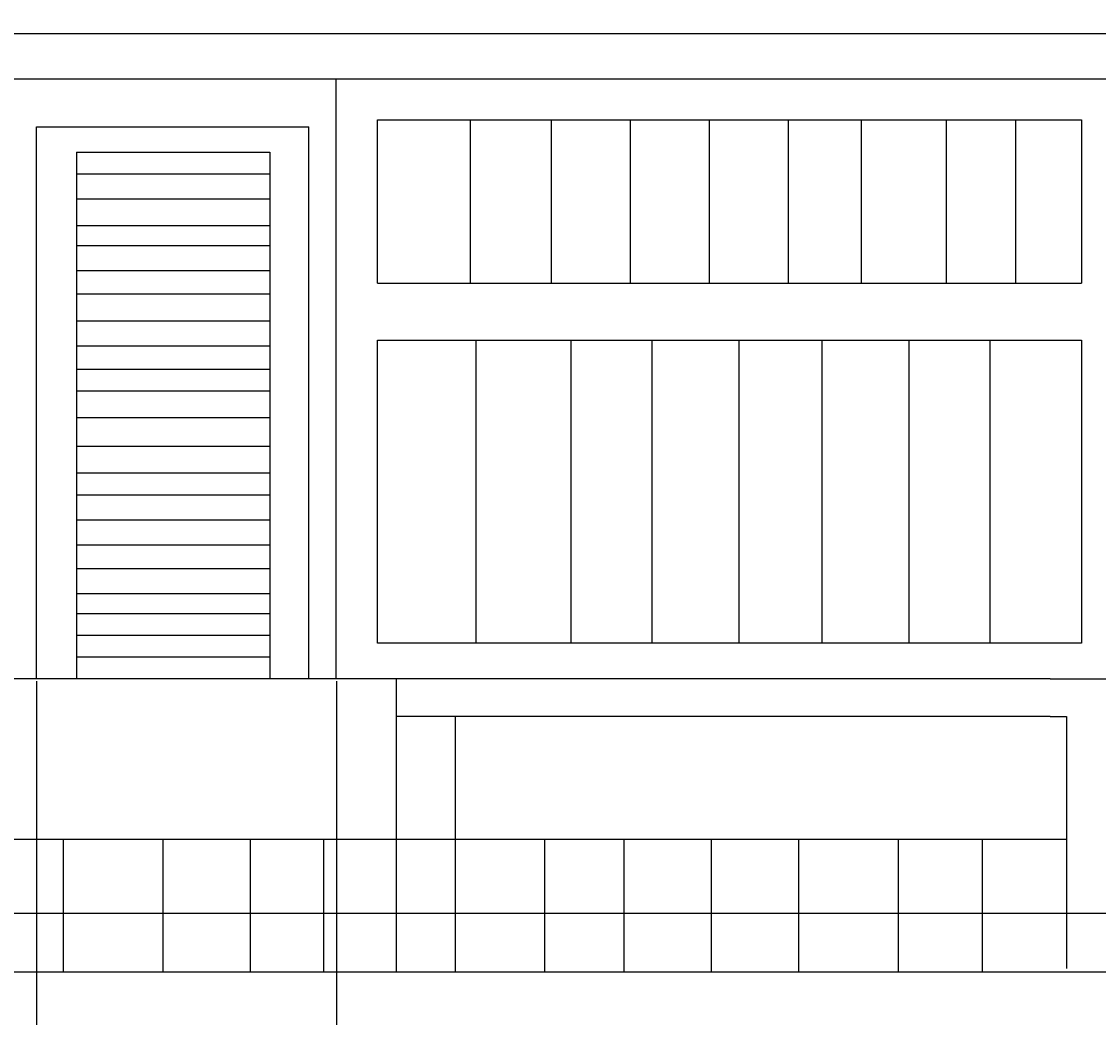
# Model space of a CAD drawing. Units: inches. Extents: x -117 to 121, y -77 to 40.
# Tile 7 of 45: x -73 to -46, y -48 to -23. Entities that reach past the tile are written whole.
import ezdxf

# ---------------------------------------------------------------- set-up
doc = ezdxf.new("R2010")
doc.units = ezdxf.units.IN
doc.header["$MEASUREMENT"] = 0
doc.layers.add('A-ANNO-DIMS', color=2, linetype='Continuous', lineweight=18)
doc.layers.add('A-ELEV', color=7, linetype='Continuous', lineweight=25)
doc.styles.get("Standard").update_dxf_attribs({"font": 'arial.ttf'})
doc.dimstyles.get("Standard").update_dxf_attribs({"dimtxt": 0.18, "dimasz": 0.18, "dimexe": 0.18, "dimexo": 0.0625, "dimgap": 0.09, "dimtad": 0, "dimtih": 1, "dimtoh": 1, "dimdec": 4, "dimzin": 0, "dimdsep": 46, "dimtxsty": 'Standard', "dimcen": 0.09, "dimadec": 0, "dimazin": 0, "dimtfac": 1, "dimtdec": 4, "dimtofl": 0, "dimtmove": 0, "dimatfit": 3, "dimfxl": 1, "dimtolj": 1, "dimtzin": 0, "dimarcsym": 0})

# ---------------------------------------------------------------- blocks, each defined once
blk = doc.blocks.new('*D13')
at = {"layer": 'A-ANNO-DIMS', "color": 0, "lineweight": -2, "transparency": 16777216}
for p, q in [((-2.663, 27.063), (-117.024, 27.063)), ((-116.844, 26.883), (-116.844, -16.974)), ((-116.844, -61.196), (-116.844, -17.338)), ((-106.096, -61.376), (-117.024, -61.376))]:
    blk.add_line(p, q, dxfattribs=at)
at = {"layer": 'A-ANNO-DIMS', "color": 0, "transparency": 16777216}
for points in [[(-116.874, 26.883), (-116.814, 26.883), (-116.844, 27.063)], [(-116.874, -61.196), (-116.814, -61.196), (-116.844, -61.376)]]:
    blk.add_solid(points, dxfattribs=at)
at = {"layer": 'Defpoints', "color": 0, "transparency": 16777216}
for p in [(-2.6, 27.063), (-116.844, -61.376), (-106.034, -61.376)]:
    blk.add_point(p, dxfattribs=at)
at = {"layer": 'A-ANNO-DIMS', "color": 0, "transparency": 16777216, "insert": (-116.844, -17.156), "char_height": 0.18, "attachment_point": 5}
blk.add_mtext('\\A1;88.44', dxfattribs=at)
blk = doc.blocks.new('*D37')
at = {"layer": 'A-ANNO-DIMS', "color": 0, "lineweight": -2, "transparency": 16777216}
for p, q in [((-3.912, -45.613), (-117.024, -45.613)), ((-116.844, -45.793), (-116.844, -52.47)), ((-116.844, -59.512), (-116.844, -52.834)), ((-3.912, -59.692), (-117.024, -59.692))]:
    blk.add_line(p, q, dxfattribs=at)
at = {"layer": 'A-ANNO-DIMS', "color": 0, "transparency": 16777216}
for points in [[(-116.874, -45.793), (-116.814, -45.793), (-116.844, -45.613)], [(-116.874, -59.512), (-116.814, -59.512), (-116.844, -59.692)]]:
    blk.add_solid(points, dxfattribs=at)
at = {"layer": 'Defpoints', "color": 0, "transparency": 16777216}
for p in [(-116.844, -45.613), (-3.85, -45.613), (-3.85, -59.692)]:
    blk.add_point(p, dxfattribs=at)
at = {"layer": 'A-ANNO-DIMS', "color": 0, "transparency": 16777216, "insert": (-116.844, -52.652), "char_height": 0.18, "attachment_point": 5}
blk.add_mtext('\\A1;14.079', dxfattribs=at)
blk = doc.blocks.new('*D46')
at = {"layer": 'A-ANNO-DIMS', "color": 0, "lineweight": -2, "transparency": 16777216}
for p, q in [((-78.307, -39.778), (-78.307, -77.193)), ((-72.705, -39.778), (-72.705, -77.193)), ((-78.127, -77.013), (-75.882, -77.013)), ((-72.885, -77.013), (-75.13, -77.013))]:
    blk.add_line(p, q, dxfattribs=at)
at = {"layer": 'A-ANNO-DIMS', "color": 0, "transparency": 16777216}
for points in [[(-78.127, -76.983), (-78.127, -77.043), (-78.307, -77.013)], [(-72.885, -76.983), (-72.885, -77.043), (-72.705, -77.013)]]:
    blk.add_solid(points, dxfattribs=at)
at = {"layer": 'Defpoints', "color": 0, "transparency": 16777216}
for p in [(-78.307, -39.716), (-72.705, -39.716), (-72.705, -77.013)]:
    blk.add_point(p, dxfattribs=at)
at = {"layer": 'A-ANNO-DIMS', "color": 0, "transparency": 16777216, "insert": (-75.506, -77.013), "char_height": 0.18, "attachment_point": 5}
blk.add_mtext('\\A1;5.601', dxfattribs=at)
blk = doc.blocks.new('*D47')
at = {"layer": 'A-ANNO-DIMS', "color": 0, "lineweight": -2, "transparency": 16777216}
for p, q in [((-72.705, -39.778), (-72.705, -77.193)), ((-65.167, -39.778), (-65.167, -77.193)), ((-72.525, -77.013), (-69.329, -77.013)), ((-65.347, -77.013), (-68.543, -77.013))]:
    blk.add_line(p, q, dxfattribs=at)
at = {"layer": 'A-ANNO-DIMS', "color": 0, "transparency": 16777216}
for points in [[(-72.525, -76.983), (-72.525, -77.043), (-72.705, -77.013)], [(-65.347, -76.983), (-65.347, -77.043), (-65.167, -77.013)]]:
    blk.add_solid(points, dxfattribs=at)
at = {"layer": 'Defpoints', "color": 0, "transparency": 16777216}
for p in [(-72.705, -39.716), (-65.167, -39.716), (-65.167, -77.013)]:
    blk.add_point(p, dxfattribs=at)
at = {"layer": 'A-ANNO-DIMS', "color": 0, "transparency": 16777216, "insert": (-68.936, -77.013), "char_height": 0.18, "attachment_point": 5}
blk.add_mtext('\\A1;7.538', dxfattribs=at)
blk = doc.blocks.new('*D48')
at = {"layer": 'A-ANNO-DIMS', "color": 0, "lineweight": -2, "transparency": 16777216}
for p, q in [((-65.167, -39.778), (-65.167, -77.193)), ((-45.533, -39.778), (-45.533, -77.193)), ((-64.987, -77.013), (-55.805, -77.013)), ((-45.713, -77.013), (-54.895, -77.013))]:
    blk.add_line(p, q, dxfattribs=at)
at = {"layer": 'A-ANNO-DIMS', "color": 0, "transparency": 16777216}
for points in [[(-64.987, -76.983), (-64.987, -77.043), (-65.167, -77.013)], [(-45.713, -76.983), (-45.713, -77.043), (-45.533, -77.013)]]:
    blk.add_solid(points, dxfattribs=at)
at = {"layer": 'Defpoints', "color": 0, "transparency": 16777216}
for p in [(-65.167, -39.716), (-45.533, -39.716), (-45.533, -77.013)]:
    blk.add_point(p, dxfattribs=at)
at = {"layer": 'A-ANNO-DIMS', "color": 0, "transparency": 16777216, "insert": (-55.35, -77.013), "char_height": 0.18, "attachment_point": 5}
blk.add_mtext('\\A1;19.634', dxfattribs=at)

msp = doc.modelspace()

# ---------------------------------------------------------------- linework, layer by layer
at = {"layer": 'A-ELEV'}
for p, q in [((-45.4848, -23.5007), (-94.4355, -23.5007)), ((-78.1044, -24.6358), (-45.4848, -24.6358)), ((-65.1673, -39.716), (-65.1673, -24.6358)), ((-64.1321, -25.6604), (-46.437, -25.6604)), ((-64.1321, -29.7655), (-64.1321, -25.6604)), ((-61.7982, -29.7655), (-61.7982, -25.6604)), ((-59.7622, -29.7655), (-59.7622, -25.6604)), ((-57.7759, -29.7655), (-57.7759, -25.6604)), ((-55.7896, -29.7655), (-55.7896, -25.6604)), ((-53.8033, -29.7655), (-53.8033, -25.6604)), ((-51.9659, -29.7655), (-51.9659, -25.6604)), ((-49.8307, -29.7655), (-49.8307, -25.6604)), ((-48.0926, -29.7655), (-48.0926, -25.6604)), ((-46.437, -25.6604), (-46.437, -29.7655)), ((-72.7053, -39.716), (-72.7053, -25.8422)), ((-72.7053, -25.8422), (-65.8588, -25.8422)), ((-71.6931, -25.8422), (-66.8375, -25.8422)), ((-65.8588, -39.716), (-65.8588, -25.8422)), ((-71.6931, -26.4721), (-66.8375, -26.4721)), ((-71.6931, -26.4721), (-71.6931, -39.716)), ((-66.8375, -26.4721), (-66.8375, -39.716)), ((-71.6931, -27.018), (-66.8375, -27.018)), ((-71.6931, -27.648), (-66.8375, -27.648)), ((-71.6931, -28.3199), (-66.8375, -28.3199)), ((-71.6931, -28.8238), (-66.8375, -28.8238)), ((-71.6931, -29.4537), (-66.8375, -29.4537)), ((-64.1321, -29.7655), (-46.437, -29.7655)), ((-71.6931, -30.0416), (-66.8375, -30.0416)), ((-71.6931, -30.7136), (-66.8375, -30.7136)), ((-71.6931, -31.3435), (-66.8375, -31.3435)), ((-64.1321, -38.817), (-64.1321, -31.2038)), ((-64.1321, -31.2038), (-46.437, -31.2038)), ((-61.6492, -38.817), (-61.6492, -31.2038)), ((-59.2656, -38.817), (-59.2656, -31.2038)), ((-57.2297, -38.817), (-57.2297, -31.2038)), ((-55.0447, -38.817), (-55.0447, -31.2038)), ((-52.9591, -38.817), (-52.9591, -31.2038)), ((-50.7742, -38.817), (-50.7742, -31.2038)), ((-48.7382, -38.817), (-48.7382, -31.2038)), ((-46.437, -31.2038), (-46.437, -38.817)), ((-71.6931, -31.9314), (-66.8375, -31.9314)), ((-71.6931, -32.4773), (-66.8375, -32.4773)), ((-71.6931, -33.1492), (-66.8375, -33.1492)), ((-71.6931, -33.8631), (-66.8375, -33.8631)), ((-71.6931, -34.5351), (-66.8375, -34.5351)), ((-71.6931, -35.0909), (-66.8375, -35.0909)), ((-71.6931, -35.7208), (-66.8375, -35.7208)), ((-71.6931, -36.3507), (-66.8375, -36.3507)), ((-71.6931, -36.9386), (-66.8375, -36.9386)), ((-71.6931, -37.5685), (-66.8375, -37.5685)), ((-71.6931, -38.0725), (-66.8375, -38.0725)), ((-71.6931, -38.6184), (-66.8375, -38.6184)), ((-46.437, -38.817), (-64.1321, -38.817)), ((-71.6931, -39.1643), (-66.8375, -39.1643)), ((-63.664, -39.716), (-87.0424, -39.716)), ((-47.2265, -39.716), (-63.664, -39.716)), ((-63.664, -39.716), (-63.664, -47.0788)), ((-47.2265, -39.716), (-22.8601, -39.716)), ((-47.2265, -40.6605), (-63.664, -40.6605)), ((-62.1811, -40.6605), (-62.1811, -47.0788)), ((-47.2265, -40.6605), (-46.814, -40.6605)), ((-46.814, -40.6605), (-46.814, -46.9969)), ((-74.3335, -43.7463), (-46.814, -43.7463)), ((-72.0236, -47.0788), (-72.0236, -43.7463)), ((-69.518, -47.0788), (-69.518, -43.7463)), ((-67.3255, -47.0788), (-67.3255, -43.7463)), ((-65.4854, -47.0788), (-65.4854, -43.7463)), ((-59.926, -47.0788), (-59.926, -43.7463)), ((-57.9294, -47.0788), (-57.9294, -43.7463)), ((-55.7369, -47.0788), (-55.7369, -43.7463)), ((-53.5445, -47.0788), (-53.5445, -43.7463)), ((-51.0388, -47.0788), (-51.0388, -43.7463)), ((-48.9247, -47.0788), (-48.9247, -43.7463)), ((-74.3335, -47.0788), (-22.8601, -47.0788))]:
    msp.add_line(p, q, dxfattribs=at)

# ---------------------------------------------------------------- dimensions: what is measured, and where the dimension line sits
at = {"layer": 'A-ANNO-DIMS'}
for base, p1, p2, override, picture, middle in [((-116.8438, -61.3756), (-2.6001, 27.0634), (-106.0338, -61.3756), {"dimdec": 2, "dimlfac": 1, "dimrnd": 0, "dimzin": 0, "dimdsep": 46, "dimlunit": 2}, '*D13', (-116.8438, -17.1561)), ((-116.843772, -45.612514), (-3.849514, -59.692012), (-3.849514, -45.612514), {"dimdec": 3, "dimlfac": 1, "dimrnd": 0, "dimzin": 0, "dimdsep": 46, "dimlunit": 2}, '*D37', (-116.843772, -52.652263))]:
    dim = msp.add_linear_dim(base=base, p1=p1, p2=p2, angle=90, dimstyle='Standard', override=override, dxfattribs=at)
    dim.commit()
    dim.dimension.update_dxf_attribs({"geometry": picture, "text_midpoint": middle})
for base, p1, p2, picture, middle in [((-72.70528, -77.01347), (-78.30676, -39.71597), (-72.70528, -39.71597), '*D46', (-75.50602, -77.01347)), ((-65.1673, -77.0135), (-72.7053, -39.716), (-65.1673, -39.716), '*D47', (-68.9363, -77.0135)), ((-45.5331, -77.0135), (-65.1673, -39.716), (-45.5331, -39.716), '*D48', (-55.3502, -77.0135))]:
    dim = msp.add_linear_dim(base=base, p1=p1, p2=p2, dimstyle='Standard', override={"dimdec": 3, "dimlfac": 1, "dimrnd": 0, "dimzin": 0, "dimdsep": 46, "dimlunit": 2}, dxfattribs=at)
    dim.commit()
    dim.dimension.update_dxf_attribs({"geometry": picture, "text_midpoint": middle})

doc.saveas('drawing.dxf')
